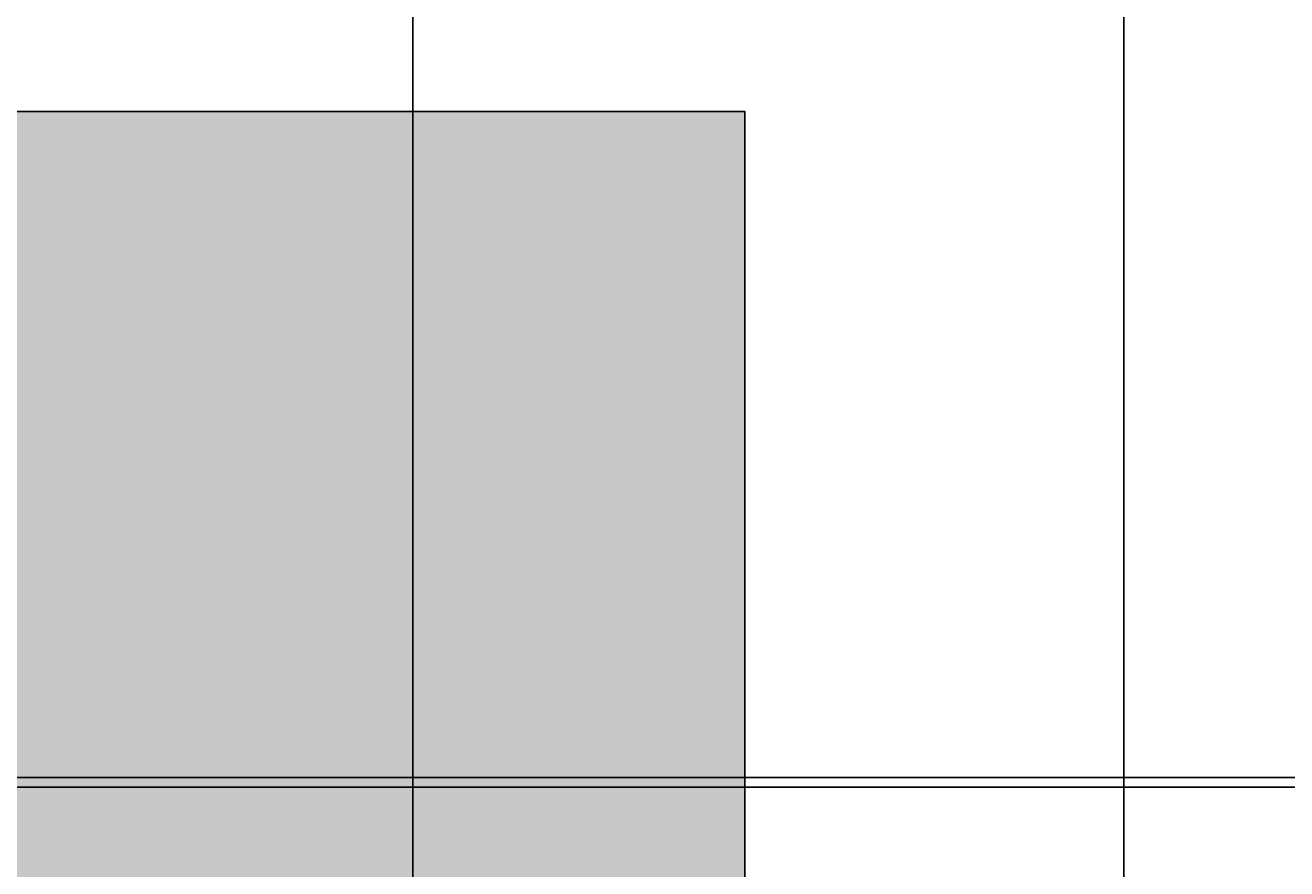
# Model space of a CAD drawing. Units: inches. Extents: x 35362 to 73946, y 43607 to 67532.
# Tile 69 of 134: x 47763 to 48464, y 49269 to 49738. Entities that reach past the tile are written whole.
import ezdxf

# ---------------------------------------------------------------- set-up
doc = ezdxf.new("R2010")
doc.units = ezdxf.units.IN
doc.header["$MEASUREMENT"] = 0
for name, color, linetype, lineweight in [('A-ANNO-DIMS', 2, 'Continuous', 18), ('E-SYMB', 1, 'Continuous', 25), ('E-SYMB-PATT', 1, 'Continuous', 13)]:
    doc.layers.add(name, color=color, linetype=linetype, lineweight=lineweight)
doc.styles.get("Standard").update_dxf_attribs({"font": 'arial.ttf'})
doc.dimstyles.get("Standard").update_dxf_attribs({"dimtxt": 0.18, "dimasz": 0.18, "dimexe": 0.18, "dimexo": 0.0625, "dimgap": 0.09, "dimtad": 0, "dimtih": 1, "dimtoh": 1, "dimdec": 4, "dimzin": 0, "dimdsep": 46, "dimtxsty": 'Standard', "dimcen": 0.09, "dimadec": 0, "dimazin": 0, "dimtfac": 1, "dimtdec": 4, "dimtofl": 0, "dimtmove": 0, "dimatfit": 3, "dimfxl": 1, "dimtolj": 1, "dimtzin": 0, "dimarcsym": 0})

# ---------------------------------------------------------------- blocks, each defined once
blk = doc.blocks.new('*D11')
at = {"layer": 'A-ANNO-DIMS', "color": 0, "lineweight": -2, "transparency": 16777216}
for p, q in [((47978.66, 56028.77), (47978.66, 43606.68)), ((53109.76, 56028.77), (53109.76, 43606.68)), ((47978.84, 43606.86), (50543.87, 43606.86)), ((53109.58, 43606.86), (50544.55, 43606.86))]:
    blk.add_line(p, q, dxfattribs=at)
at = {"layer": 'A-ANNO-DIMS', "color": 0, "transparency": 16777216}
for points in [[(47978.84, 43606.89), (47978.84, 43606.83), (47978.66, 43606.86)], [(53109.58, 43606.89), (53109.58, 43606.83), (53109.76, 43606.86)]]:
    blk.add_solid(points, dxfattribs=at)
at = {"layer": 'Defpoints', "color": 0, "transparency": 16777216}
for p in [(47978.66, 56028.84), (53109.76, 56028.84), (53109.76, 43606.86)]:
    blk.add_point(p, dxfattribs=at)
at = {"layer": 'A-ANNO-DIMS', "color": 0, "transparency": 16777216, "insert": (50544.21, 43606.86), "char_height": 0.18, "attachment_point": 5}
blk.add_mtext('\\A1;5131', dxfattribs=at)
blk = doc.blocks.new('*D13')
at = {"layer": 'A-ANNO-DIMS', "color": 0, "lineweight": -2, "transparency": 16777216}
for p, q in [((48373.49, 51694.02), (48373.49, 43606.68)), ((51029.04, 51694.02), (51029.04, 43606.68)), ((48373.67, 43606.86), (49700.8, 43606.86)), ((51028.86, 43606.86), (49701.73, 43606.86))]:
    blk.add_line(p, q, dxfattribs=at)
at = {"layer": 'A-ANNO-DIMS', "color": 0, "transparency": 16777216}
for points in [[(48373.67, 43606.89), (48373.67, 43606.83), (48373.49, 43606.86)], [(51028.86, 43606.89), (51028.86, 43606.83), (51029.04, 43606.86)]]:
    blk.add_solid(points, dxfattribs=at)
at = {"layer": 'Defpoints', "color": 0, "transparency": 16777216}
for p in [(48373.49, 51694.09), (51029.04, 51694.09), (51029.04, 43606.86)]:
    blk.add_point(p, dxfattribs=at)
at = {"layer": 'A-ANNO-DIMS', "color": 0, "transparency": 16777216, "insert": (49701.27, 43606.86), "char_height": 0.18, "attachment_point": 5}
blk.add_mtext('\\A1;2655.6', dxfattribs=at)
blk = doc.blocks.new('*D27')
at = {"layer": 'A-ANNO-DIMS', "color": 0, "lineweight": -2, "transparency": 16777216}
for p, q in [((47978.66, 56028.77), (47978.66, 43606.68)), ((48373.49, 53428.96), (48373.49, 43606.68)), ((47978.84, 43606.86), (48175.68, 43606.86)), ((48373.31, 43606.86), (48176.47, 43606.86))]:
    blk.add_line(p, q, dxfattribs=at)
at = {"layer": 'A-ANNO-DIMS', "color": 0, "transparency": 16777216}
for points in [[(47978.84, 43606.89), (47978.84, 43606.83), (47978.66, 43606.86)], [(48373.31, 43606.89), (48373.31, 43606.83), (48373.49, 43606.86)]]:
    blk.add_solid(points, dxfattribs=at)
at = {"layer": 'Defpoints', "color": 0, "transparency": 16777216}
for p in [(47978.66, 56028.84), (48373.49, 53429.02), (48373.49, 43606.86)]:
    blk.add_point(p, dxfattribs=at)
at = {"layer": 'A-ANNO-DIMS', "color": 0, "transparency": 16777216, "insert": (48176.08, 43606.86), "char_height": 0.18, "attachment_point": 5}
blk.add_mtext('\\A1;394.8', dxfattribs=at)
blk = doc.blocks.new('*D40')
at = {"layer": 'A-ANNO-DIMS', "color": 0, "lineweight": -2, "transparency": 16777216}
for p, q in [((56873.54, 53351.53), (35361.77, 53351.53)), ((35361.95, 53351.35), (35361.95, 51333.28)), ((35361.95, 49314.85), (35361.95, 51332.92)), ((51806.45, 49314.67), (35361.77, 49314.67))]:
    blk.add_line(p, q, dxfattribs=at)
at = {"layer": 'A-ANNO-DIMS', "color": 0, "transparency": 16777216}
for points in [[(35361.92, 53351.35), (35361.98, 53351.35), (35361.95, 53351.53)], [(35361.92, 49314.85), (35361.98, 49314.85), (35361.95, 49314.67)]]:
    blk.add_solid(points, dxfattribs=at)
at = {"layer": 'Defpoints', "color": 0, "transparency": 16777216}
for p in [(35361.95, 53351.53), (56873.6, 53351.53), (51806.52, 49314.67)]:
    blk.add_point(p, dxfattribs=at)
at = {"layer": 'A-ANNO-DIMS', "color": 0, "transparency": 16777216, "insert": (35361.95, 51333.1), "char_height": 0.18, "attachment_point": 5}
blk.add_mtext('\\A1;4036.9', dxfattribs=at)
blk = doc.blocks.new('*D67')
at = {"layer": 'A-ANNO-DIMS', "color": 0, "lineweight": -2, "transparency": 16777216}
for p, q in [((56873.54, 53351.53), (35361.77, 53351.53)), ((35361.95, 53351.35), (35361.95, 49400.89)), ((35361.95, 45450.07), (35361.95, 49400.53)), ((53793.58, 45449.89), (35361.77, 45449.89))]:
    blk.add_line(p, q, dxfattribs=at)
at = {"layer": 'A-ANNO-DIMS', "color": 0, "transparency": 16777216}
for points in [[(35361.92, 53351.35), (35361.98, 53351.35), (35361.95, 53351.53)], [(35361.92, 45450.07), (35361.98, 45450.07), (35361.95, 45449.89)]]:
    blk.add_solid(points, dxfattribs=at)
at = {"layer": 'Defpoints', "color": 0, "transparency": 16777216}
for p in [(35361.95, 53351.53), (56873.6, 53351.53), (53793.64, 45449.89)]:
    blk.add_point(p, dxfattribs=at)
at = {"layer": 'A-ANNO-DIMS', "color": 0, "transparency": 16777216, "insert": (35361.95, 49400.71), "char_height": 0.18, "attachment_point": 5}
blk.add_mtext('\\A1;7901.6', dxfattribs=at)
blk = doc.blocks.new('*D86')
at = {"layer": 'A-ANNO-DIMS', "color": 0, "lineweight": -2, "transparency": 16777216}
for p, q in [((51285.53, 49320.08), (35361.77, 49320.08)), ((35361.95, 49319.9), (35361.95, 49120.26)), ((35361.95, 48920.26), (35361.95, 49119.9)), ((51285.53, 48920.08), (35361.77, 48920.08))]:
    blk.add_line(p, q, dxfattribs=at)
at = {"layer": 'A-ANNO-DIMS', "color": 0, "transparency": 16777216}
for points in [[(35361.92, 49319.9), (35361.98, 49319.9), (35361.95, 49320.08)], [(35361.92, 48920.26), (35361.98, 48920.26), (35361.95, 48920.08)]]:
    blk.add_solid(points, dxfattribs=at)
at = {"layer": 'Defpoints', "color": 0, "transparency": 16777216}
for p in [(35361.95, 49320.08), (51285.59, 49320.08), (51285.59, 48920.08)]:
    blk.add_point(p, dxfattribs=at)
at = {"layer": 'A-ANNO-DIMS', "color": 0, "transparency": 16777216, "insert": (35361.95, 49120.08), "char_height": 0.18, "attachment_point": 5}
blk.add_mtext('\\A1;400.0', dxfattribs=at)

msp = doc.modelspace()

# ---------------------------------------------------------------- hatches: boundary and pattern name
at = {"layer": 'E-SYMB-PATT'}
h = msp.add_hatch(color=256, dxfattribs=at)
h.dxf.hatch_style = 1
h.paths.add_polyline_path([(48163.038, 49689.843), (45390.147, 49689.843), (45390.147, 46919.381), (48163.038, 46919.381)])

# ---------------------------------------------------------------- linework, layer by layer
at = {"layer": 'E-SYMB'}
msp.add_lwpolyline([(45390.147, 49689.843), (48163.038, 49689.843), (48163.038, 46919.381), (45390.147, 46919.381)], close=True, dxfattribs=at)

# ---------------------------------------------------------------- dimensions: what is measured, and where the dimension line sits
at = {"layer": 'A-ANNO-DIMS'}
for base, p1, p2, override, picture, middle in [((53109.76, 43606.859), (47978.665, 56028.836), (53109.76, 56028.836), {"dimdec": 0, "dimlfac": 1, "dimrnd": 0, "dimzin": 0, "dimdsep": 46, "dimlunit": 2}, '*D11', (50544.212, 43606.859)), ((48373.492, 43606.859), (47978.665, 56028.836), (48373.492, 53429.019), {"dimdec": 1, "dimlfac": 1, "dimrnd": 0, "dimzin": 0, "dimdsep": 46, "dimlunit": 2}, '*D27', (48176.078, 43606.859)), ((51029.043, 43606.859), (48373.492, 51694.087), (51029.043, 51694.087), {"dimdec": 1, "dimlfac": 1, "dimrnd": 0, "dimzin": 0, "dimdsep": 46, "dimlunit": 2}, '*D13', (49701.267, 43606.859))]:
    dim = msp.add_linear_dim(base=base, p1=p1, p2=p2, dimstyle='Standard', override=override, dxfattribs=at)
    dim.commit()
    dim.dimension.update_dxf_attribs({"geometry": picture, "text_midpoint": middle})
for base, p1, p2, picture, middle in [((35361.949, 53351.529), (51806.517, 49314.669), (56873.602, 53351.529), '*D40', (35361.949, 51333.099)), ((35361.949, 53351.529), (53793.638, 45449.894), (56873.602, 53351.529), '*D67', (35361.949, 49400.712)), ((35361.949, 49320.079), (51285.595, 48920.079), (51285.595, 49320.079), '*D86', (35361.949, 49120.079))]:
    dim = msp.add_linear_dim(base=base, p1=p1, p2=p2, angle=90, dimstyle='Standard', override={"dimdec": 1, "dimlfac": 1, "dimrnd": 0, "dimzin": 0, "dimdsep": 46, "dimlunit": 2}, dxfattribs=at)
    dim.commit()
    dim.dimension.update_dxf_attribs({"geometry": picture, "text_midpoint": middle})

doc.saveas('drawing.dxf')
